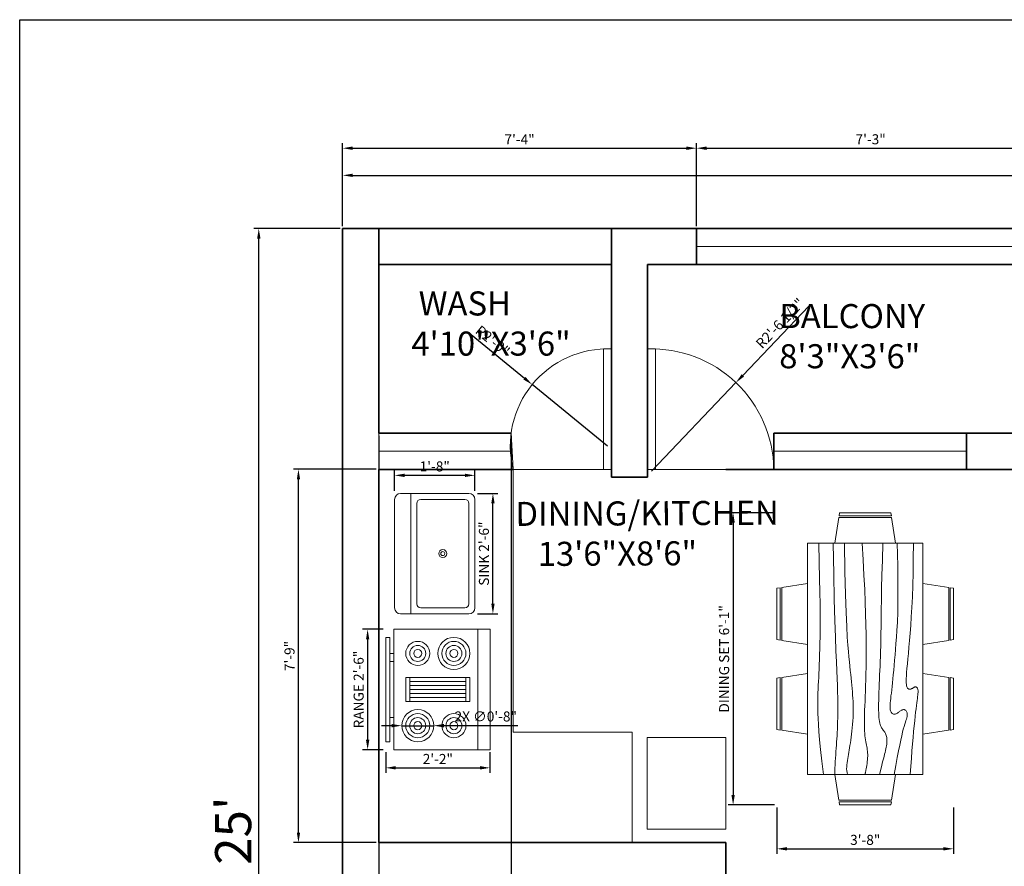
# Model space of a CAD drawing. Units: inches. Extents: x 5717 to 6221, y 11359 to 11763.
# Tile 2 of 4: x 5717 to 5963, y 11552 to 11763. Entities that reach past the tile are written whole.
import ezdxf

# ---------------------------------------------------------------- set-up
doc = ezdxf.new("R2010")
doc.units = ezdxf.units.IN
for name, color, linetype, lineweight, true_color in [('A-ANNO-DIMS', 254, 'Continuous', 13, 0xfeeab9), ('A-ANNO-TTLB', 51, 'Continuous', 25, 0xf8f6b0), ('A-AREA-IDEN', 11, 'Continuous', 20, 0xf27172), ('A-FLOR-CASE', 244, 'Continuous', 20, 0x991b1e), ('A-WALL', 244, 'Continuous', 35, 0x991b1e)]:
    doc.layers.add(name, color=color, linetype=linetype, lineweight=lineweight, true_color=true_color)
for name, color, linetype, lineweight in [('A-DOOR', 5, 'Continuous', 18), ('A-EQPM', 8, 'Continuous', 18), ('A-FLOR-FIXT', 1, 'Continuous', 18), ('A-FURN', 8, 'Continuous', 18), ('A-GLAZ', 4, 'Continuous', 18)]:
    doc.layers.add(name, color=color, linetype=linetype, lineweight=lineweight)
doc.styles.get("Standard").update_dxf_attribs({"font": 'arial.ttf'})
doc.dimstyles.new('ISO-25', dxfattribs={"dimtxt": 2.5, "dimasz": 2.5, "dimexe": 1.25, "dimexo": 0.625, "dimtad": 1, "dimlunit": 3, "dimtxsty": 'Standard', "dimcen": 2.5, "dimadec": 0, "dimazin": 0, "dimtfac": 1, "dimtmove": 0, "dimatfit": 3, "dimfxl": 1, "dimarcsym": 0})

# ---------------------------------------------------------------- blocks, each defined once
blk = doc.blocks.new('*D12')
at = {"layer": 'A-ANNO-DIMS', "color": 0, "lineweight": -2, "transparency": 16777216}
for p, q in [((5797.9, 11711.73), (5797.9, 11725.6)), ((6157.9, 11711.73), (6157.9, 11725.6)), ((5800.4, 11724.35), (6155.4, 11724.35))]:
    blk.add_line(p, q, dxfattribs=at)
at = {"layer": 'A-ANNO-DIMS', "color": 0, "transparency": 16777216}
for points in [[(5800.4, 11724.77), (5800.4, 11723.94), (5797.9, 11724.35)], [(6155.4, 11724.77), (6155.4, 11723.94), (6157.9, 11724.35)]]:
    blk.add_solid(points, dxfattribs=at)
at = {"layer": 'Defpoints', "color": 0, "transparency": 16777216}
for p in [(6157.9, 11724.35), (5797.9, 11711.11), (6157.9, 11711.11)]:
    blk.add_point(p, dxfattribs=at)
at = {"layer": 'A-ANNO-DIMS', "color": 0, "transparency": 16777216, "insert": (5977.9, 11729.58), "char_height": 9, "attachment_point": 5}
blk.add_mtext("30'", dxfattribs=at)
blk = doc.blocks.new('*D13')
at = {"layer": 'A-ANNO-DIMS', "color": 0, "lineweight": -2, "transparency": 16777216}
for p, q in [((5797.28, 11711.11), (5775.76, 11711.11)), ((5777.01, 11413.61), (5777.01, 11708.61)), ((5797.28, 11411.11), (5775.76, 11411.11))]:
    blk.add_line(p, q, dxfattribs=at)
at = {"layer": 'A-ANNO-DIMS', "color": 0, "transparency": 16777216}
for points in [[(5776.6, 11708.61), (5777.43, 11708.61), (5777.01, 11711.11)], [(5776.6, 11413.61), (5777.43, 11413.61), (5777.01, 11411.11)]]:
    blk.add_solid(points, dxfattribs=at)
at = {"layer": 'Defpoints', "color": 0, "transparency": 16777216}
for p in [(5777.01, 11711.11), (5797.9, 11711.11), (5797.9, 11411.11)]:
    blk.add_point(p, dxfattribs=at)
at = {"layer": 'A-ANNO-DIMS', "color": 0, "transparency": 16777216, "insert": (5771.79, 11561.11), "char_height": 9, "attachment_point": 5, "rotation": 90}
blk.add_mtext("25'", dxfattribs=at)
blk = doc.blocks.new('Dining Set - 36 x 72 in.')
for p, q in [((-22.2343, 26.00059), (-23.4847, 17.99762)), ((-22.2304, 26), (-5.7608, 26)), ((-22, 27.5), (-22.1562, 26.50042)), ((-5.8416, 26.5), (-22.1534, 26.5)), ((-22, 27.5), (-6, 27.5)), ((-5.8437, 26.49966), (-6, 27.5)), ((-4.5152, 17.99762), (-5.7655, 25.99926)), ((5.7657, 26.00059), (4.5153, 17.99762)), ((5.7696, 26), (22.2392, 26)), ((6, 27.5), (5.8438, 26.50042)), ((22.1584, 26.5), (5.8466, 26.5)), ((6, 27.5), (22, 27.5)), ((22.1563, 26.49966), (22, 27.5)), ((23.4848, 17.99762), (22.2345, 25.99926)), ((36, 18), (-36, 18)), ((-36, 18), (-36, -18)), ((36, -18), (36, 18)), ((-44.0006, 8.23428), (-35.9976, 9.48474)), ((44.0006, 8.23428), (35.9976, 9.48474)), ((-45.5, 8), (-44.5004, 8.15617)), ((-45.5, 8), (-45.5, -8)), ((-44.5, -8.15843), (-44.5, 8.15338)), ((-44, 8.23041), (-44, -8.23915)), ((44, 8.23041), (44, -8.23915)), ((44.5, -8.15843), (44.5, 8.15338)), ((45.5, 8), (44.5005, 8.15617)), ((45.5, 8), (45.5, -8)), ((-44.4997, -8.15631), (-45.5, -8)), ((-35.9976, -9.48476), (-43.9993, -8.2345)), ((35.9976, -9.48476), (43.9993, -8.2345)), ((44.4997, -8.15631), (45.5, -8)), ((-36, -18), (36, -18)), ((-22.2343, -26.0006), (-23.4847, -17.99762)), ((-4.5152, -17.99762), (-5.7655, -25.99928)), ((5.7657, -26.0006), (4.5153, -17.99762)), ((23.4848, -17.99762), (22.2345, -25.99928)), ((-22.2304, -26), (-5.7608, -26)), ((-22, -27.5), (-22.1562, -26.50044)), ((-5.8416, -26.5), (-22.1534, -26.5)), ((-22, -27.5), (-6, -27.5)), ((-5.8437, -26.49967), (-6, -27.5)), ((5.7696, -26), (22.2392, -26)), ((6, -27.5), (5.8438, -26.50044)), ((22.1584, -26.5), (5.8466, -26.5)), ((6, -27.5), (22, -27.5)), ((22.1563, -26.49967), (22, -27.5))]:
    blk.add_line(p, q)
for points in [[(-36, 15), (-31.1772, 14.97754), (-26.8079, 14.91406), (-22.8538, 14.81543), (-19.276, 14.6875), (-16.0362, 14.53613), (-13.0957, 14.36718), (-10.4159, 14.18652), (-7.9583, 14), (-5.6904, 13.81315), (-3.6035, 13.63021), (-1.6954, 13.45508), (0.0365, 13.29166), (1.5945, 13.14388), (2.9811, 13.01562), (4.1988, 12.9108), (5.25, 12.83333), (6.1393, 12.78613), (6.8802, 12.76823), (7.4883, 12.77767), (7.9792, 12.8125), (8.3685, 12.87077), (8.6719, 12.95052), (8.9049, 13.0498), (9.0833, 13.16666), (9.2205, 13.29899), (9.3216, 13.44401), (9.3895, 13.59879), (9.4271, 13.76041), (9.4373, 13.92594), (9.4232, 14.09245), (9.3875, 14.257), (9.3333, 14.41666), (9.2638, 14.56917), (9.1836, 14.71484), (9.0975, 14.85465), (9.0104, 14.98958), (8.9272, 15.1206), (8.8529, 15.2487), (8.7922, 15.37483), (8.75, 15.5), (8.7305, 15.62467), (8.7344, 15.74739), (8.7617, 15.86621), (8.8125, 15.97916), (8.8867, 16.08431), (8.9844, 16.17968), (9.1055, 16.26334), (9.25, 16.33333), (9.4189, 16.38802), (9.6172, 16.42708), (9.8506, 16.45052), (10.125, 16.45833), (10.4463, 16.45052), (10.8203, 16.42708), (11.2529, 16.38802), (11.75, 16.33333), (12.3184, 16.26318), (12.9694, 16.17838), (13.7151, 16.07991), (14.5677, 15.96875), (15.5395, 15.84586), (16.6426, 15.71224), (17.8893, 15.56884), (19.2917, 15.41666), (20.859, 15.25667), (22.5879, 15.08984), (24.4721, 14.91715), (26.5052, 14.73958), (28.6809, 14.5581), (30.9929, 14.3737), (33.4347, 14.18733), (36, 14)], [(-36, 10), (-28.9766, 10.14274), (-23.1725, 10.20442), (-18.4241, 10.19775), (-14.5677, 10.13541), (-11.4399, 10.03011), (-8.877, 9.89453), (-6.7154, 9.74137), (-4.7917, 9.58333), (-2.9698, 9.43082), (-1.2246, 9.28515), (0.4415, 9.14534), (2.026, 9.01041), (3.5266, 8.87939), (4.9408, 8.7513), (6.266, 8.62516), (7.5, 8.5), (8.6411, 8.37549), (9.6914, 8.2539), (10.6538, 8.13818), (11.5312, 8.03125), (12.3267, 7.93603), (13.043, 7.85547), (13.6831, 7.79248), (14.25, 7.75), (14.7471, 7.7303), (15.1797, 7.73307), (15.5537, 7.75732), (15.875, 7.80208), (16.1494, 7.86637), (16.3828, 7.94922), (16.5811, 8.04964), (16.75, 8.16666), (16.8944, 8.29915), (17.0143, 8.44531), (17.1089, 8.60319), (17.1771, 8.77083), (17.218, 8.94629), (17.2305, 9.1276), (17.2137, 9.31282), (17.1667, 9.5), (17.0895, 9.6875), (16.987, 9.875), (16.8649, 10.0625), (16.7292, 10.25), (16.5856, 10.4375), (16.4401, 10.625), (16.2985, 10.8125), (16.1667, 11), (16.05, 11.18733), (15.9518, 11.3737), (15.8752, 11.5581), (15.8229, 11.73958), (15.798, 11.91715), (15.8034, 12.08984), (15.842, 12.25667), (15.9167, 12.41666), (16.0295, 12.56836), (16.1784, 12.70833), (16.3605, 12.83268), (16.5729, 12.9375), (16.8127, 13.01888), (17.0768, 13.07291), (17.3625, 13.0957), (17.6667, 13.08333), (17.9894, 13.03312), (18.3418, 12.94726), (18.7382, 12.82918), (19.1927, 12.68229), (19.7195, 12.51001), (20.3327, 12.31575), (21.0465, 12.10294), (21.875, 11.875), (22.8357, 11.63354), (23.959, 11.37304), (25.2786, 11.08618), (26.8282, 10.76562), (28.6414, 10.40405), (30.752, 9.99414), (33.1936, 9.52856), (36, 9)], [(-36, 5.5), (-30.7157, 5.3348), (-26.069, 5.20963), (-21.9946, 5.11767), (-18.4271, 5.05208), (-15.3009, 5.00602), (-12.5508, 4.97265), (-10.1112, 4.94515), (-7.9167, 4.91666), (-5.909, 4.88167), (-4.0586, 4.83984), (-2.3429, 4.79215), (-0.7396, 4.73958), (0.7739, 4.6831), (2.22, 4.6237), (3.6213, 4.56233), (5, 4.5), (6.373, 4.43782), (7.7344, 4.3776), (9.0723, 4.32129), (10.375, 4.27083), (11.6309, 4.22819), (12.8281, 4.19531), (13.9551, 4.17415), (15, 4.16666), (15.954, 4.17448), (16.819, 4.19791), (17.6001, 4.23698), (18.3021, 4.29166), (18.9299, 4.36198), (19.4883, 4.44791), (19.9823, 4.54948), (20.4167, 4.66666), (20.7969, 4.79899), (21.1302, 4.94401), (21.4245, 5.09879), (21.6875, 5.26041), (21.9271, 5.42594), (22.1511, 5.59245), (22.3672, 5.757), (22.5834, 5.91666), (22.8065, 6.06868), (23.0404, 6.21093), (23.2879, 6.34147), (23.5521, 6.45833), (23.8358, 6.55957), (24.142, 6.64323), (24.4735, 6.70735), (24.8334, 6.75), (25.2235, 6.76969), (25.642, 6.76692), (26.0858, 6.74267), (26.5521, 6.69791), (27.0379, 6.63362), (27.5404, 6.55078), (28.0565, 6.45036), (28.5834, 6.33333), (29.1242, 6.19987), (29.7071, 6.04687), (30.3661, 5.87044), (31.1354, 5.66666), (32.0493, 5.43164), (33.142, 5.16146), (34.4475, 4.85221), (36, 4.5)], [(-36, -1), (-30.7915, -0.6591), (-26.0195, -0.38216), (-21.6519, -0.16284), (-17.6563, 0.00521), (-14.0005, 0.12833), (-10.6523, 0.21289), (-7.5796, 0.26522), (-4.75, 0.29166), (-2.134, 0.29793), (0.2878, 0.28711), (2.5317, 0.26163), (4.6146, 0.22396), (6.5529, 0.17651), (8.3633, 0.12174), (10.0623, 0.06209), (11.6667, 0), (13.1899, -0.06201), (14.6341, -0.1211), (15.9982, -0.17432), (17.2813, -0.21875), (18.4823, -0.25147), (19.6003, -0.26953), (20.6343, -0.27002), (21.5834, -0.25), (22.4481, -0.20768), (23.2357, -0.14584), (23.9549, -0.06836), (24.6146, 0.02083), (25.2235, 0.11784), (25.7904, 0.21875), (26.3241, 0.31966), (26.8334, 0.41666), (27.3265, 0.50618), (27.8099, 0.58593), (28.2894, 0.65397), (28.7709, 0.70833), (29.2601, 0.74707), (29.763, 0.76823), (30.2855, 0.76985), (30.8334, 0.75), (31.4088, 0.70784), (31.9994, 0.64713), (32.589, 0.57275), (33.1615, 0.48958), (33.7008, 0.4025), (34.1908, 0.3164), (34.6153, 0.23616), (34.9584, 0.16666), (35.2099, 0.11165), (35.3848, 0.07031), (35.504, 0.04069), (35.5886, 0.02083), (35.6594, 0.00879), (35.7377, 0.0026), (35.8442, 0.00032), (36, 0)], [(-36, -6.5), (-27.1843, -6.31267), (-20.084, -6.1263), (-14.469, -5.9419), (-10.1094, -5.76042), (-6.7752, -5.58285), (-4.2363, -5.41016), (-2.2629, -5.24333), (-0.625, -5.08334), (0.8708, -4.93099), (2.2715, -4.78646), (3.5872, -4.64974), (4.8281, -4.52084), (6.0046, -4.39974), (7.127, -4.28646), (8.2053, -4.18099), (9.25, -4.08334), (10.2705, -3.99382), (11.2734, -3.91407), (12.2647, -3.84603), (13.25, -3.79167), (14.2354, -3.75293), (15.2266, -3.73177), (16.2295, -3.73015), (17.25, -3.75), (18.2912, -3.79248), (19.3451, -3.85547), (20.4009, -3.93604), (21.4479, -4.03125), (22.4754, -4.13819), (23.4727, -4.25391), (24.4289, -4.37549), (25.3334, -4.5), (26.1785, -4.62492), (26.9694, -4.74935), (27.7145, -4.87281), (28.4219, -4.99479), (29.1, -5.11483), (29.7572, -5.23242), (30.4016, -5.34709), (31.0417, -5.45834), (31.6837, -5.56437), (32.3262, -5.65821), (32.9658, -5.73153), (33.599, -5.77604), (34.2224, -5.78345), (34.8327, -5.74545), (35.4264, -5.65373), (36, -5.5)], [(-36, -10), (-26.4022, -9.81299), (-18.4675, -9.62891), (-11.9839, -9.45069), (-6.7396, -9.28125), (-2.5226, -9.12354), (0.8789, -8.98047), (3.6769, -8.85498), (6.0833, -8.75), (8.2767, -8.66765), (10.3021, -8.60677), (12.1712, -8.56543), (13.8958, -8.54167), (15.4876, -8.53353), (16.9583, -8.53907), (18.3197, -8.55632), (19.5834, -8.58334), (20.7616, -8.61841), (21.8685, -8.66081), (22.9188, -8.71004), (23.9271, -8.76563), (24.9081, -8.82707), (25.8763, -8.89388), (26.8465, -8.96558), (27.8334, -9.04167), (28.8474, -9.12118), (29.8828, -9.20117), (30.93, -9.27824), (31.9792, -9.34896), (33.0205, -9.40991), (34.0443, -9.45768), (35.0407, -9.48885), (36, -9.5)], [(-36, -14.5), (-30.0881, -14.33513), (-25.0332, -14.21224), (-20.7312, -14.12647), (-17.0781, -14.07292), (-13.97, -14.04671), (-11.3027, -14.04297), (-8.9724, -14.05681), (-6.875, -14.08334), (-4.9224, -14.11833), (-3.0905, -14.16016), (-1.3709, -14.20785), (0.2448, -14.26042), (1.7647, -14.3169), (3.1973, -14.3763), (4.5507, -14.43767), (5.8333, -14.5), (7.0554, -14.5621), (8.235, -14.62175), (9.3922, -14.67652), (10.5469, -14.72396), (11.7192, -14.76164), (12.929, -14.78711), (14.1965, -14.79794), (15.5417, -14.79167), (16.9933, -14.76424), (18.6152, -14.70508), (20.4804, -14.60197), (22.6615, -14.44271), (25.2312, -14.21509), (28.2624, -13.9069), (31.8277, -13.50594), (36, -13)]]:
    blk.add_lwpolyline(points)
blk = doc.blocks.new('Range-Oven - 30 in top')
for p, q in [((0, -3), (30, -3)), ((12, -6), (18, -6)), ((13, -20), (13, -6)), ((14, -6), (14, -20)), ((15, -20), (15, -6)), ((16, -6), (16, -20)), ((17, -20), (17, -6)), ((18, -20), (12, -20)), ((6, -24), (6, -25)), ((8, -25), (8, -24)), ((22, -25), (22, -24)), ((24, -24), (24, -25))]:
    blk.add_line(p, q)
for points in [[(0, -24), (0, 0), (30, 0), (30, -24)], [(12, -21), (12, -5), (18, -5), (18, -21)], [(2, -26), (2, -25), (28, -25), (28, -26)]]:
    blk.add_lwpolyline(points, close=True)
for centre, radius in [((6, -9), 4), ((6, -9), 3), ((6, -9), 2), ((24, -9), 3), ((24, -9), 2), ((6, -9), 1), ((24, -9), 1), ((24, -18), 4), ((6, -18), 3), ((6, -18), 2), ((6, -18), 1), ((24, -18), 3), ((24, -18), 2), ((24, -18), 1)]:
    blk.add_circle(centre, radius)
blk = doc.blocks.new('Sink-single - 30 in top')
blk.add_line((-15, -3.999996), (15, -3.999996))
for points in [[(-13.5, 0), (13.5, 0)], [(-15, -18.499996), (-15, -1.5)], [(15, -1.5), (15, -18.499996)], [(-13.5, -17.499996), (-13.5, -6.499996)], [(-12.5, -5.499996), (12.5, -5.499996)], [(13.5, -6.499996), (13.5, -17.499996)], [(12.5, -18.499996), (-12.5, -18.499996)], [(13.5, -19.999996), (-13.5, -19.999996)]]:
    blk.add_lwpolyline(points)
for radius in [1, 0.5]:
    blk.add_circle((0, -11.999996), radius)
for centre, radius, start, end in [((-13.5, -1.5), 1.5, 90, 180), ((13.5, -1.5), 1.5, 0, 90), ((-12.5, -6.499996), 1, 90, 180), ((12.5, -6.499996), 1, 0, 90), ((-13.5, -18.499996), 1.5, 180, 270), ((-12.5, -17.499996), 1, 180, 270), ((12.5, -17.499996), 1, 270, 0), ((13.5, -18.499996), 1.5, 270, 0)]:
    blk.add_arc(centre, radius, start, end)
blk = doc.blocks.new('DOOR-LEAF-30IN')
for p, q in [((2, 30), (0, 30)), ((0, 30), (0, 0)), ((2, 0), (2, 30))]:
    blk.add_line(p, q)
blk = doc.blocks.new('WIN-48IN')
for p, q in [((0, 0), (0, 9)), ((0, 9), (48, 9)), ((48, 9), (48, 0)), ((0, 4.5), (48, 4.5)), ((48, 0), (0, 0))]:
    blk.add_line(p, q)
blk = doc.blocks.new('*D32')
at = {"layer": 'A-ANNO-DIMS', "color": 0, "lineweight": -2, "transparency": 16777216}
for p, q in [((5905.53, 11640.29), (5893.99, 11640.29)), ((5895.24, 11637.79), (5895.24, 11569.99)), ((5905.53, 11567.49), (5893.99, 11567.49))]:
    blk.add_line(p, q, dxfattribs=at)
at = {"layer": 'A-ANNO-DIMS', "color": 0, "transparency": 16777216}
for points in [[(5894.82, 11637.79), (5895.65, 11637.79), (5895.24, 11640.29)], [(5894.82, 11569.99), (5895.65, 11569.99), (5895.24, 11567.49)]]:
    blk.add_solid(points, dxfattribs=at)
at = {"layer": 'Defpoints', "color": 0, "transparency": 16777216}
for p in [(5906.16, 11640.29), (5895.24, 11567.49), (5906.16, 11567.49)]:
    blk.add_point(p, dxfattribs=at)
at = {"layer": 'A-ANNO-DIMS', "color": 0, "transparency": 16777216, "insert": (5893.32, 11603.89), "char_height": 2.5, "attachment_point": 5, "rotation": 90}
blk.add_mtext('DINING SET 6\'-1"', dxfattribs=at)
blk = doc.blocks.new('*D33')
at = {"layer": 'A-ANNO-DIMS', "color": 0, "lineweight": -2, "transparency": 16777216}
for p, q in [((5906.16, 11566.87), (5906.16, 11555.32)), ((5950.16, 11566.87), (5950.16, 11555.32)), ((5908.66, 11556.57), (5947.66, 11556.57))]:
    blk.add_line(p, q, dxfattribs=at)
at = {"layer": 'A-ANNO-DIMS', "color": 0, "transparency": 16777216}
for points in [[(5908.66, 11556.99), (5908.66, 11556.15), (5906.16, 11556.57)], [(5947.66, 11556.99), (5947.66, 11556.15), (5950.16, 11556.57)]]:
    blk.add_solid(points, dxfattribs=at)
at = {"layer": 'Defpoints', "color": 0, "transparency": 16777216}
for p in [(5906.16, 11567.49), (5950.16, 11567.49), (5950.16, 11556.57)]:
    blk.add_point(p, dxfattribs=at)
at = {"layer": 'A-ANNO-DIMS', "color": 0, "transparency": 16777216, "insert": (5928.16, 11558.47), "char_height": 2.5, "attachment_point": 5}
blk.add_mtext('3\'-8"', dxfattribs=at)
blk = doc.blocks.new('*D34')
at = {"layer": 'A-ANNO-DIMS', "color": 0, "lineweight": -2, "transparency": 16777216}
for p, q in [((5808.02, 11611.25), (5802.89, 11611.25)), ((5804.14, 11608.75), (5804.14, 11583.75)), ((5808.02, 11581.25), (5802.89, 11581.25))]:
    blk.add_line(p, q, dxfattribs=at)
at = {"layer": 'A-ANNO-DIMS', "color": 0, "transparency": 16777216}
for points in [[(5803.73, 11608.75), (5804.56, 11608.75), (5804.14, 11611.25)], [(5803.73, 11583.75), (5804.56, 11583.75), (5804.14, 11581.25)]]:
    blk.add_solid(points, dxfattribs=at)
at = {"layer": 'Defpoints', "color": 0, "transparency": 16777216}
for p in [(5808.64, 11611.25), (5804.14, 11581.25), (5808.64, 11581.25)]:
    blk.add_point(p, dxfattribs=at)
at = {"layer": 'A-ANNO-DIMS', "color": 0, "transparency": 16777216, "insert": (5802.23, 11596.25), "char_height": 2.5, "attachment_point": 5, "rotation": 90}
blk.add_mtext('RANGE 2\'-6"', dxfattribs=at)
blk = doc.blocks.new('*D35')
at = {"layer": 'A-ANNO-DIMS', "color": 0, "lineweight": -2, "transparency": 16777216}
for p, q in [((5808.64, 11580.63), (5808.64, 11575.5)), ((5834.64, 11580.63), (5834.64, 11575.5)), ((5811.14, 11576.75), (5832.14, 11576.75))]:
    blk.add_line(p, q, dxfattribs=at)
at = {"layer": 'A-ANNO-DIMS', "color": 0, "transparency": 16777216}
for points in [[(5811.14, 11577.17), (5811.14, 11576.33), (5808.64, 11576.75)], [(5832.14, 11577.17), (5832.14, 11576.33), (5834.64, 11576.75)]]:
    blk.add_solid(points, dxfattribs=at)
at = {"layer": 'Defpoints', "color": 0, "transparency": 16777216}
for p in [(5808.64, 11581.25), (5834.64, 11581.25), (5834.64, 11576.75)]:
    blk.add_point(p, dxfattribs=at)
at = {"layer": 'A-ANNO-DIMS', "color": 0, "transparency": 16777216, "insert": (5821.64, 11578.63), "char_height": 2.5, "attachment_point": 5}
blk.add_mtext('2\'-2"', dxfattribs=at)
blk = doc.blocks.new('*D36')
at = {"layer": 'A-ANNO-DIMS', "color": 0, "lineweight": -2, "transparency": 16777216}
for p, q in [((5831.5, 11645.11), (5836.62, 11645.11)), ((5835.37, 11617.61), (5835.37, 11642.61)), ((5831.5, 11615.11), (5836.62, 11615.11))]:
    blk.add_line(p, q, dxfattribs=at)
at = {"layer": 'A-ANNO-DIMS', "color": 0, "transparency": 16777216}
for points in [[(5834.96, 11642.61), (5835.79, 11642.61), (5835.37, 11645.11)], [(5834.96, 11617.61), (5835.79, 11617.61), (5835.37, 11615.11)]]:
    blk.add_solid(points, dxfattribs=at)
at = {"layer": 'Defpoints', "color": 0, "transparency": 16777216}
for p in [(5830.87, 11645.11), (5835.37, 11645.11), (5830.87, 11615.11)]:
    blk.add_point(p, dxfattribs=at)
at = {"layer": 'A-ANNO-DIMS', "color": 0, "transparency": 16777216, "insert": (5833.45, 11630.11), "char_height": 2.5, "attachment_point": 5, "rotation": 90}
blk.add_mtext('SINK 2\'-6"', dxfattribs=at)
blk = doc.blocks.new('*D37')
at = {"layer": 'A-ANNO-DIMS', "color": 0, "lineweight": -2, "transparency": 16777216}
for p, q in [((5810.87, 11645.74), (5810.87, 11650.86)), ((5828.37, 11649.61), (5813.37, 11649.61)), ((5830.87, 11645.74), (5830.87, 11650.86))]:
    blk.add_line(p, q, dxfattribs=at)
at = {"layer": 'A-ANNO-DIMS', "color": 0, "transparency": 16777216}
for points in [[(5813.37, 11650.03), (5813.37, 11649.19), (5810.87, 11649.61)], [(5828.37, 11650.03), (5828.37, 11649.19), (5830.87, 11649.61)]]:
    blk.add_solid(points, dxfattribs=at)
at = {"layer": 'Defpoints', "color": 0, "transparency": 16777216}
for p in [(5810.87, 11649.61), (5810.87, 11645.11), (5830.87, 11645.11)]:
    blk.add_point(p, dxfattribs=at)
at = {"layer": 'A-ANNO-DIMS', "color": 0, "transparency": 16777216, "insert": (5820.87, 11651.51), "char_height": 2.5, "attachment_point": 5}
blk.add_mtext('1\'-8"', dxfattribs=at)
blk = doc.blocks.new('*D49')
at = {"layer": 'A-ANNO-DIMS', "color": 0, "lineweight": -2, "transparency": 16777216}
for p, q in [((5806.28, 11651.11), (5785.65, 11651.11)), ((5786.9, 11560.61), (5786.9, 11648.61)), ((5806.28, 11558.11), (5785.65, 11558.11))]:
    blk.add_line(p, q, dxfattribs=at)
at = {"layer": 'A-ANNO-DIMS', "color": 0, "transparency": 16777216}
for points in [[(5786.49, 11648.61), (5787.32, 11648.61), (5786.9, 11651.11)], [(5786.49, 11560.61), (5787.32, 11560.61), (5786.9, 11558.11)]]:
    blk.add_solid(points, dxfattribs=at)
at = {"layer": 'Defpoints', "color": 0, "transparency": 16777216}
for p in [(5786.9, 11651.11), (5806.9, 11651.11), (5806.9, 11558.11)]:
    blk.add_point(p, dxfattribs=at)
at = {"layer": 'A-ANNO-DIMS', "color": 0, "transparency": 16777216, "insert": (5785, 11604.61), "char_height": 2.5, "attachment_point": 5, "rotation": 90}
blk.add_mtext('7\'-9"', dxfattribs=at)
blk = doc.blocks.new('*D50')
at = {"layer": 'A-ANNO-DIMS', "color": 0, "lineweight": -2, "transparency": 16777216}
for p, q in [((5797.9, 11711.73), (5797.9, 11732.36)), ((5800.4, 11731.11), (5883.61, 11731.11)), ((5886.11, 11711.73), (5886.11, 11732.36))]:
    blk.add_line(p, q, dxfattribs=at)
at = {"layer": 'A-ANNO-DIMS', "color": 0, "transparency": 16777216}
for points in [[(5800.4, 11731.53), (5800.4, 11730.69), (5797.9, 11731.11)], [(5883.61, 11731.53), (5883.61, 11730.69), (5886.11, 11731.11)]]:
    blk.add_solid(points, dxfattribs=at)
at = {"layer": 'Defpoints', "color": 0, "transparency": 16777216}
for p in [(5886.11, 11731.11), (5797.9, 11711.11), (5886.11, 11711.11)]:
    blk.add_point(p, dxfattribs=at)
at = {"layer": 'A-ANNO-DIMS', "color": 0, "transparency": 16777216, "insert": (5842.01, 11732.98), "char_height": 2.5, "attachment_point": 5}
blk.add_mtext('7\'-4"', dxfattribs=at)
blk = doc.blocks.new('*D51')
at = {"layer": 'A-ANNO-DIMS', "color": 0, "lineweight": -2, "transparency": 16777216}
for p, q in [((5886.11, 11711.73), (5886.11, 11732.36)), ((5888.61, 11731.11), (5970.4, 11731.11)), ((5972.9, 11711.73), (5972.9, 11732.36))]:
    blk.add_line(p, q, dxfattribs=at)
at = {"layer": 'A-ANNO-DIMS', "color": 0, "transparency": 16777216}
for points in [[(5888.61, 11731.53), (5888.61, 11730.69), (5886.11, 11731.11)], [(5970.4, 11731.53), (5970.4, 11730.69), (5972.9, 11731.11)]]:
    blk.add_solid(points, dxfattribs=at)
at = {"layer": 'Defpoints', "color": 0, "transparency": 16777216}
for p in [(5972.9, 11731.11), (5886.11, 11711.11), (5972.9, 11711.11)]:
    blk.add_point(p, dxfattribs=at)
at = {"layer": 'A-ANNO-DIMS', "color": 0, "transparency": 16777216, "insert": (5929.51, 11733.01), "char_height": 2.5, "attachment_point": 5}
blk.add_mtext('7\'-3"', dxfattribs=at)
blk = doc.blocks.new('*D56')
at = {"layer": 'A-ANNO-DIMS', "color": 0, "lineweight": -2, "transparency": 16777216}
for p, q in [((5806.9, 11659.48), (5806.9, 11389.86)), ((5839.9, 11659.48), (5839.9, 11389.86)), ((5809.4, 11391.11), (5837.4, 11391.11))]:
    blk.add_line(p, q, dxfattribs=at)
at = {"layer": 'A-ANNO-DIMS', "color": 0, "transparency": 16777216}
for points in [[(5809.4, 11391.53), (5809.4, 11390.69), (5806.9, 11391.11)], [(5837.4, 11391.53), (5837.4, 11390.69), (5839.9, 11391.11)]]:
    blk.add_solid(points, dxfattribs=at)
at = {"layer": 'Defpoints', "color": 0, "transparency": 16777216}
for p in [(5806.9, 11660.11), (5839.9, 11660.11), (5839.9, 11391.11)]:
    blk.add_point(p, dxfattribs=at)
at = {"layer": 'A-ANNO-DIMS', "color": 0, "transparency": 16777216, "insert": (5823.4, 11393.01), "char_height": 2.5, "attachment_point": 5}
blk.add_mtext('2\'-9"', dxfattribs=at)
blk = doc.blocks.new('*D63')
at = {"layer": 'A-ANNO-DIMS', "color": 0, "lineweight": -2, "transparency": 16777216}
for p, q in [((5914.11, 11691.78), (5897.66, 11674.52)), ((5874.9, 11650.64), (5895.93, 11672.71))]:
    blk.add_line(p, q, dxfattribs=at)
at = {"layer": 'A-ANNO-DIMS', "color": 0, "transparency": 16777216}
blk.add_solid([(5897.36, 11674.81), (5897.96, 11674.23), (5895.93, 11672.71)], dxfattribs=at)
at = {"layer": 'Defpoints', "color": 0, "transparency": 16777216}
for p in [(5895.93, 11672.71), (5874.9, 11650.64)]:
    blk.add_point(p, dxfattribs=at)
at = {"layer": 'A-ANNO-DIMS', "color": 0, "transparency": 16777216, "insert": (5907.16, 11687.27), "char_height": 2.5, "attachment_point": 5, "rotation": 46.3758}
blk.add_mtext('R2\'-6 1/2"', dxfattribs=at)
blk = doc.blocks.new('*D65')
at = {"layer": 'A-ANNO-DIMS', "color": 0, "lineweight": -2, "transparency": 16777216}
for p, q in [((5829.92, 11684.68), (5843.22, 11673.82)), ((5863.9, 11656.92), (5845.15, 11672.23))]:
    blk.add_line(p, q, dxfattribs=at)
at = {"layer": 'A-ANNO-DIMS', "color": 0, "transparency": 16777216}
blk.add_solid([(5843.48, 11674.14), (5842.95, 11673.49), (5845.15, 11672.23)], dxfattribs=at)
at = {"layer": 'Defpoints', "color": 0, "transparency": 16777216}
for p in [(5845.15, 11672.23), (5863.9, 11656.92)]:
    blk.add_point(p, dxfattribs=at)
at = {"layer": 'A-ANNO-DIMS', "color": 0, "transparency": 16777216, "insert": (5835.1, 11682.89), "char_height": 2.5, "attachment_point": 5, "rotation": 320.7629}
blk.add_mtext('R2\'-0"', dxfattribs=at)
blk = doc.blocks.new('*D72')
at = {"layer": 'A-ANNO-DIMS', "color": 0, "lineweight": -2, "transparency": 16777216}
for p, q in [((5810.14, 11587.25), (5807.64, 11587.25)), ((5812.64, 11587.25), (5820.64, 11587.25)), ((5841.54, 11587.25), (5823.14, 11587.25))]:
    blk.add_line(p, q, dxfattribs=at)
at = {"layer": 'A-ANNO-DIMS', "color": 0, "transparency": 16777216}
for points in [[(5810.14, 11587.67), (5810.14, 11586.83), (5812.64, 11587.25)], [(5823.14, 11587.67), (5823.14, 11586.83), (5820.64, 11587.25)]]:
    blk.add_solid(points, dxfattribs=at)
at = {"layer": 'Defpoints', "color": 0, "transparency": 16777216}
for p in [(5812.64, 11587.25), (5820.64, 11587.25)]:
    blk.add_point(p, dxfattribs=at)
at = {"layer": 'A-ANNO-DIMS', "color": 0, "transparency": 16777216, "insert": (5833.59, 11589.22), "char_height": 2.5, "attachment_point": 5, "rotation": 0.0021}
blk.add_mtext('2X ∅0\'-8"', dxfattribs=at)

msp = doc.modelspace()

# ---------------------------------------------------------------- linework, layer by layer
at = {"layer": 'A-ANNO-TTLB'}
msp.add_lwpolyline([(5717.423, 11763.126), (6221.432, 11763.126), (6221.432, 11381.867), (5717.423, 11381.867)], close=True, dxfattribs=at)
at = {"layer": 'A-DOOR'}
for p, q in [((5840.402, 11651.109), (5864.902, 11651.109)), ((5840.402, 11651.109), (5862.902, 11651.109)), ((5862.902, 11651.109), (5840.402, 11651.109)), ((5873.902, 11651.109), (5893.38, 11651.109)), ((5893.38, 11651.109), (5873.902, 11651.109)), ((5893.38, 11651.109), (5905.38, 11651.109)), ((5893.38, 11651.109), (5905.38, 11651.109)), ((5905.38, 11651.109), (5905.38, 11651.109)), ((5905.38, 11651.109), (5905.38, 11651.109))]:
    msp.add_line(p, q, dxfattribs=at)
for centre, radius, start, end in [((5863.902, 11656.921), 24.208, 87.63253, 193.89274), ((5874.902, 11650.644), 30.481, 0.87316, 91.88006)]:
    msp.add_arc(centre, radius, start, end, dxfattribs=at)
at = {"layer": 'A-FLOR-CASE'}
for p, q in [((5822.616, 11651.109), (5840.402, 11651.109)), ((5840.402, 11651.109), (5840.402, 11585.619)), ((5840.402, 11585.619), (5870.07, 11585.619)), ((5870.07, 11585.619), (5870.07, 11558.109))]:
    msp.add_line(p, q, dxfattribs=at)
msp.add_lwpolyline([(5873.853, 11584.287), (5893.38, 11584.287), (5893.38, 11561.44), (5873.853, 11561.44)], close=True, dxfattribs=at)
at = {"layer": 'A-GLAZ'}
for p, q in [((5806.902, 11702.109), (5806.902, 11711.109)), ((5864.902, 11711.109), (5806.902, 11711.109)), ((5864.902, 11702.109), (5864.902, 11711.109)), ((5864.902, 11702.109), (5864.902, 11711.109)), ((5886.109, 11702.109), (5886.109, 11711.109)), ((5886.109, 11711.109), (5972.902, 11711.109)), ((5886.109, 11706.609), (5972.902, 11706.609)), ((5806.902, 11702.109), (5864.902, 11702.109)), ((5972.902, 11702.109), (5886.109, 11702.109)), ((5806.902, 11660.109), (5806.902, 11651.109)), ((5839.905, 11660.109), (5806.902, 11660.109)), ((5840.402, 11651.109), (5839.905, 11660.109)), ((5806.902, 11655.609), (5840.154, 11655.609)), ((5806.902, 11651.109), (5840.402, 11651.109))]:
    msp.add_line(p, q, dxfattribs=at)
at = {"layer": 'A-WALL'}
for p, q in [((5797.902, 11711.109), (5797.902, 11462.109)), ((6157.902, 11711.109), (5797.902, 11711.109)), ((5806.902, 11702.109), (5806.902, 11711.109)), ((5864.902, 11711.109), (5864.902, 11651.109)), ((5864.902, 11702.109), (5864.902, 11711.109)), ((5886.109, 11702.109), (5886.109, 11711.109)), ((5806.902, 11702.109), (5806.902, 11660.109)), ((5864.902, 11702.109), (5806.902, 11702.109)), ((5873.902, 11702.109), (5873.902, 11651.109)), ((5972.902, 11702.109), (5873.902, 11702.109)), ((5839.905, 11660.109), (5806.902, 11660.109)), ((5972.902, 11660.109), (5905.38, 11660.109)), ((5905.38, 11660.109), (5905.38, 11651.109)), ((5953.38, 11660.109), (5953.38, 11651.109)), ((5806.902, 11651.109), (5806.902, 11558.109)), ((5840.402, 11651.109), (5806.902, 11651.109)), ((5864.902, 11651.109), (5864.902, 11649.184)), ((5873.902, 11649.184), (5873.902, 11651.109)), ((5972.902, 11651.109), (5893.38, 11651.109)), ((5864.902, 11649.184), (5873.902, 11649.184)), ((5873.902, 11558.109), (5806.902, 11558.109)), ((5873.902, 11558.109), (5861.902, 11558.109)), ((5873.902, 11558.109), (5893.38, 11558.109)), ((5893.38, 11558.109), (5893.38, 11549.109))]:
    msp.add_line(p, q, dxfattribs=at)

# ---------------------------------------------------------------- block references
at = {"layer": 'A-DOOR'}
for p in [(5862.902, 11651.109), (5873.902, 11651.109)]:
    msp.add_blockref('DOOR-LEAF-30IN', p, dxfattribs=at)
at = {"layer": 'A-EQPM', "rotation": 270}
msp.add_blockref('Range-Oven - 30 in top', (5834.643, 11611.251), dxfattribs=at)
at = {"layer": 'A-FLOR-FIXT', "rotation": 90}
msp.add_blockref('Sink-single - 30 in top', (5810.872, 11630.11), dxfattribs=at)
at = {"layer": 'A-FURN', "xscale": 0.8, "yscale": 0.8, "zscale": 0.8, "rotation": 270}
msp.add_blockref('Dining Set - 36 x 72 in.', (5928.158, 11603.89), dxfattribs=at)
at = {"layer": 'A-GLAZ'}
msp.add_blockref('WIN-48IN', (5905.38, 11651.109), dxfattribs=at)

# ---------------------------------------------------------------- texts
at = {"layer": 'A-AREA-IDEN', "char_height": 6, "attachment_point": 1}
for s, insert in [(' WASH\\P4\'10"X3\'6"', (5815.035, 11695.438)), ('  BALCONY\\P  8\'3"X3\'6"', (5903.057, 11692.281))]:
    msp.add_mtext_dynamic_manual_height_columns(s, width=116.60264, gutter_width=12.5, heights=[0], dxfattribs=dict(at, insert=insert))
at = {"layer": 'A-AREA-IDEN', "insert": (5837.308, 11642.987), "char_height": 6, "attachment_point": 1, "rotation": 0.26777}
msp.add_mtext_dynamic_manual_height_columns('  DINING/KITCHEN  \\P     13\'6"X8\'6"                   ', width=125.02015, gutter_width=12.5, heights=[41.465], dxfattribs=at)

# ---------------------------------------------------------------- dimensions: what is measured, and where the dimension line sits
at = {"layer": 'A-ANNO-DIMS'}
for base, p1, p2, override, picture, middle in [((6157.902, 11724.352), (5797.902, 11711.109), (6157.902, 11711.109), {"dimtxt": 9, "dimclrd": 0, "dimclre": 0, "dimclrt": 0}, '*D12', (5977.902, 11729.575)), ((5886.109, 11731.109), (5797.902, 11711.109), (5886.109, 11711.109), {"dimdec": 1, "dimlfac": 1, "dimrnd": 0, "dimzin": 1, "dimdsep": 46, "dimlunit": 4, "dimfrac": 2}, '*D50', (5842.006, 11732.984)), ((5972.902, 11731.109), (5886.109, 11711.109), (5972.902, 11711.109), {"dimdec": 1, "dimlfac": 1, "dimrnd": 0, "dimzin": 1, "dimdsep": 46, "dimlunit": 4, "dimfrac": 2}, '*D51', (5929.506, 11733.011)), ((5839.905, 11391.109), (5806.902, 11660.109), (5839.905, 11660.109), {"dimdec": 1, "dimlfac": 1, "dimrnd": 0, "dimzin": 1, "dimdsep": 46, "dimlunit": 4, "dimfrac": 2}, '*D56', (5823.404, 11393.01)), ((5834.643, 11576.751), (5808.643, 11581.251), (5834.643, 11581.251), {"dimdec": 1, "dimlfac": 1, "dimrnd": 0, "dimzin": 1, "dimdsep": 46, "dimlunit": 4, "dimfrac": 2}, '*D35', (5821.643, 11578.631)), ((5950.158, 11556.57), (5906.158, 11567.49), (5950.158, 11567.49), {"dimdec": 1, "dimlfac": 1, "dimrnd": 0, "dimzin": 1, "dimdsep": 46, "dimlunit": 4, "dimfrac": 2}, '*D33', (5928.158, 11558.473))]:
    dim = msp.add_linear_dim(base=base, p1=p1, p2=p2, dimstyle='ISO-25', override=override, dxfattribs=at)
    dim.commit()
    dim.dimension.update_dxf_attribs({"geometry": picture, "text_midpoint": middle})
for base, p1, p2, angle, override, picture, middle in [((5777.014, 11711.109), (5797.902, 11411.109), (5797.902, 11711.109), 90, {"dimtxt": 9, "dimclrd": 0, "dimclre": 0, "dimclrt": 0}, '*D13', (5771.794, 11561.109)), ((5810.872, 11649.61), (5830.872, 11645.11), (5810.872, 11645.11), 180, {"dimdec": 1, "dimlfac": 1, "dimrnd": 0, "dimzin": 1, "dimdsep": 46, "dimlunit": 4, "dimfrac": 2}, '*D37', (5820.872, 11651.512)), ((5786.902, 11651.109), (5806.902, 11558.109), (5806.902, 11651.109), 90, {"dimdec": 1, "dimlfac": 1, "dimrnd": 0, "dimzin": 1, "dimdsep": 46, "dimlunit": 4, "dimfrac": 2}, '*D49', (5785.001, 11604.609))]:
    dim = msp.add_linear_dim(base=base, p1=p1, p2=p2, angle=angle, dimstyle='ISO-25', override=override, dxfattribs=at)
    dim.commit()
    dim.dimension.update_dxf_attribs({"geometry": picture, "text_midpoint": middle})
for center, mpoint, picture, middle in [((5874.902, 11650.644), (5895.932, 11672.709), '*D63', (5908.55, 11685.948)), ((5863.902, 11656.921), (5845.152, 11672.234), '*D65', (5833.902, 11681.421))]:
    dim = msp.add_radius_dim(center=center, mpoint=mpoint, dimstyle='ISO-25', override={"dimdec": 1, "dimlfac": 1, "dimrnd": 0, "dimzin": 1, "dimdsep": 46, "dimlunit": 4, "dimfrac": 2}, dxfattribs=at)
    dim.commit()
    dim.dimension.update_dxf_attribs({"geometry": picture, "text_midpoint": middle, "dimtype": 164})
for base, p1, p2, angle, text, picture, middle in [((5835.372, 11645.11), (5830.872, 11615.11), (5830.872, 11645.11), 90, 'SINK <>', '*D36', (5833.455, 11630.11)), ((5895.238, 11567.49), (5906.158, 11640.29), (5906.158, 11567.49), 270, 'DINING SET <>', '*D32', (5893.32, 11603.89)), ((5804.143, 11581.251), (5808.643, 11611.251), (5808.643, 11581.251), 270, 'RANGE <>', '*D34', (5802.225, 11596.251))]:
    dim = msp.add_linear_dim(base=base, p1=p1, p2=p2, angle=angle, text=text, dimstyle='ISO-25', override={"dimdec": 1, "dimlfac": 1, "dimrnd": 0, "dimzin": 1, "dimdsep": 46, "dimlunit": 4, "dimfrac": 2}, dxfattribs=at)
    dim.commit()
    dim.dimension.update_dxf_attribs({"geometry": picture, "text_midpoint": middle})
dim = msp.add_diameter_dim_2p(p1=(5812.643, 11587.251), p2=(5820.643, 11587.251), text='2X <>', dimstyle='ISO-25', override={"dimdec": 1, "dimlfac": 1, "dimrnd": 0, "dimzin": 1, "dimdsep": 46, "dimlunit": 4, "dimfrac": 2}, dxfattribs=at)
dim.commit()
dim.dimension.update_dxf_attribs({"geometry": '*D72', "text_midpoint": (5833.591, 11587.251), "dimtype": 163})

doc.saveas('drawing.dxf')
